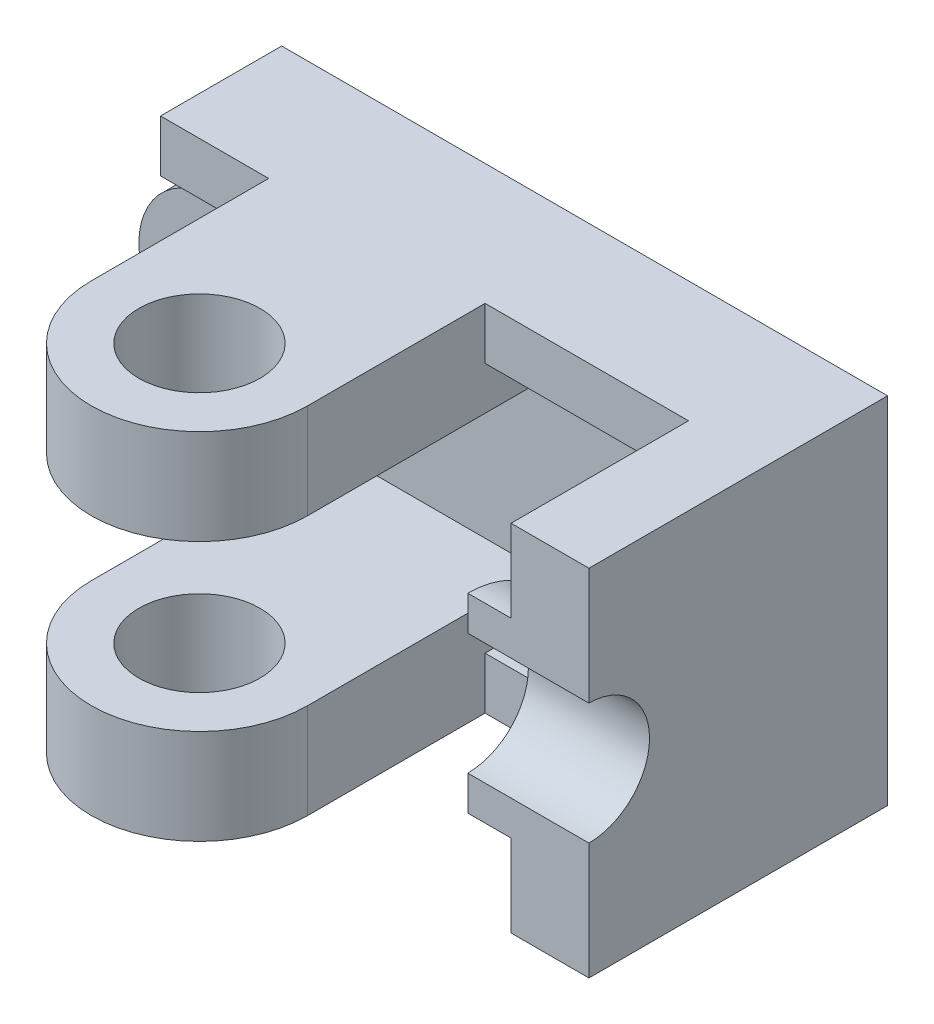
ISO-10303-21;
HEADER;
FILE_DESCRIPTION(('STEP AP214'),'2;1');
FILE_NAME('part.step','',(''),(''),'','','');
FILE_SCHEMA(('AUTOMOTIVE_DESIGN { 1 0 10303 214 1 1 1 1 }'));
ENDSEC;
DATA;
#1=APPLICATION_CONTEXT('core data for automotive mechanical design processes');
#2=APPLICATION_PROTOCOL_DEFINITION('international standard','automotive_design',2000,#1);
#3=PRODUCT_CONTEXT('',#1,'mechanical');
#4=PRODUCT('Part','Part','',(#3));
#5=PRODUCT_RELATED_PRODUCT_CATEGORY('part','',(#4));
#6=PRODUCT_DEFINITION_FORMATION('','',#4);
#7=PRODUCT_DEFINITION_CONTEXT('part definition',#1,'design');
#8=PRODUCT_DEFINITION('design','',#6,#7);
#9=PRODUCT_DEFINITION_SHAPE('','',#8);
#10=(LENGTH_UNIT() NAMED_UNIT(*) SI_UNIT(.MILLI.,.METRE.));
#11=(NAMED_UNIT(*) PLANE_ANGLE_UNIT() SI_UNIT($,.RADIAN.));
#12=(NAMED_UNIT(*) SI_UNIT($,.STERADIAN.) SOLID_ANGLE_UNIT());
#13=UNCERTAINTY_MEASURE_WITH_UNIT(LENGTH_MEASURE(1.E-05),#10,'distance_accuracy_value','');
#14=(GEOMETRIC_REPRESENTATION_CONTEXT(3) GLOBAL_UNCERTAINTY_ASSIGNED_CONTEXT((#13)) GLOBAL_UNIT_ASSIGNED_CONTEXT((#10,
#11,#12)) REPRESENTATION_CONTEXT('',''));
#15=CARTESIAN_POINT('',(0.,0.,0.));
#16=DIRECTION('',(0.,0.,1.));
#17=DIRECTION('',(1.,0.,0.));
#18=AXIS2_PLACEMENT_3D('',#15,#16,#17);
#19=CARTESIAN_POINT('',(0.,82.,15.));
#20=DIRECTION('',(1.,0.,0.));
#21=DIRECTION('',(0.,0.,-1.));
#22=AXIS2_PLACEMENT_3D('',#19,#20,#21);
#23=PLANE('',#22);
#24=DIRECTION('',(0.,-1.,0.));
#25=VECTOR('',#24,1.);
#26=CARTESIAN_POINT('',(0.,82.,0.));
#27=LINE('',#26,#25);
#28=CARTESIAN_POINT('',(0.,82.,0.));
#29=VERTEX_POINT('',#28);
#30=CARTESIAN_POINT('',(0.,59.,0.));
#31=VERTEX_POINT('',#30);
#32=EDGE_CURVE('E237',#29,#31,#27,.T.);
#33=ORIENTED_EDGE('',*,*,#32,.T.);
#34=DIRECTION('',(0.,0.,1.));
#35=VECTOR('',#34,1.);
#36=CARTESIAN_POINT('',(0.,59.,0.));
#37=LINE('',#36,#35);
#38=CARTESIAN_POINT('',(0.,59.,15.));
#39=VERTEX_POINT('',#38);
#40=EDGE_CURVE('E68',#31,#39,#37,.T.);
#41=ORIENTED_EDGE('',*,*,#40,.T.);
#42=DIRECTION('',(0.,-1.,0.));
#43=VECTOR('',#42,1.);
#44=CARTESIAN_POINT('',(0.,82.,15.));
#45=LINE('',#44,#43);
#46=CARTESIAN_POINT('',(0.,70.,15.));
#47=VERTEX_POINT('',#46);
#48=EDGE_CURVE('E439',#47,#39,#45,.T.);
#49=ORIENTED_EDGE('',*,*,#48,.F.);
#50=DIRECTION('',(0.,0.,1.));
#51=VECTOR('',#50,1.);
#52=CARTESIAN_POINT('',(0.,70.,28.));
#53=LINE('',#52,#51);
#54=CARTESIAN_POINT('',(0.,70.,28.));
#55=VERTEX_POINT('',#54);
#56=EDGE_CURVE('E257',#47,#55,#53,.T.);
#57=ORIENTED_EDGE('',*,*,#56,.T.);
#58=DIRECTION('',(0.,1.,0.));
#59=VECTOR('',#58,1.);
#60=CARTESIAN_POINT('',(0.,70.,28.));
#61=LINE('',#60,#59);
#62=CARTESIAN_POINT('',(0.,82.,28.));
#63=VERTEX_POINT('',#62);
#64=EDGE_CURVE('E269',#55,#63,#61,.T.);
#65=ORIENTED_EDGE('',*,*,#64,.T.);
#66=DIRECTION('',(0.,0.,-1.));
#67=VECTOR('',#66,1.);
#68=CARTESIAN_POINT('',(0.,82.,15.));
#69=LINE('',#68,#67);
#70=EDGE_CURVE('E441',#63,#29,#69,.T.);
#71=ORIENTED_EDGE('',*,*,#70,.T.);
#72=EDGE_LOOP('',(#33,#41,#49,#57,#65,#71));
#73=FACE_BOUND('',#72,.T.);
#74=ADVANCED_FACE('F44',(#73),#23,.F.);
#75=CARTESIAN_POINT('',(0.,0.,15.));
#76=DIRECTION('',(0.,0.,1.));
#77=DIRECTION('',(1.,0.,0.));
#78=AXIS2_PLACEMENT_3D('',#75,#76,#77);
#79=PLANE('',#78);
#80=CARTESIAN_POINT('',(0.,41.,15.));
#81=DIRECTION('',(0.,0.,1.));
#82=DIRECTION('',(1.,0.,0.));
#83=AXIS2_PLACEMENT_3D('',#80,#81,#82);
#84=CIRCLE('',#83,11.);
#85=CARTESIAN_POINT('',(11.,41.,15.));
#86=VERTEX_POINT('',#85);
#87=EDGE_CURVE('E254',#86,#86,#84,.T.);
#88=ORIENTED_EDGE('',*,*,#87,.F.);
#89=EDGE_LOOP('',(#88));
#90=FACE_BOUND('',#89,.T.);
#91=DIRECTION('',(-1.,0.,0.));
#92=VECTOR('',#91,1.);
#93=CARTESIAN_POINT('',(0.,70.,15.));
#94=LINE('',#93,#92);
#95=CARTESIAN_POINT('',(25.,70.,15.));
#96=VERTEX_POINT('',#95);
#97=EDGE_CURVE('E270',#96,#47,#94,.T.);
#98=ORIENTED_EDGE('',*,*,#97,.T.);
#99=ORIENTED_EDGE('',*,*,#48,.T.);
#100=CARTESIAN_POINT('',(0.,41.,15.));
#101=DIRECTION('',(0.,0.,1.));
#102=DIRECTION('',(1.,0.,0.));
#103=AXIS2_PLACEMENT_3D('',#100,#101,#102);
#104=CIRCLE('',#103,18.);
#105=CARTESIAN_POINT('',(0.,23.,15.));
#106=VERTEX_POINT('',#105);
#107=EDGE_CURVE('E247',#39,#106,#104,.T.);
#108=ORIENTED_EDGE('',*,*,#107,.T.);
#109=CARTESIAN_POINT('',(0.,12.,15.));
#110=VERTEX_POINT('',#109);
#111=EDGE_CURVE('E58',#106,#110,#45,.T.);
#112=ORIENTED_EDGE('',*,*,#111,.T.);
#113=DIRECTION('',(1.,0.,0.));
#114=VECTOR('',#113,1.);
#115=CARTESIAN_POINT('',(0.,12.,15.));
#116=LINE('',#115,#114);
#117=CARTESIAN_POINT('',(25.,12.,15.));
#118=VERTEX_POINT('',#117);
#119=EDGE_CURVE('E330',#110,#118,#116,.T.);
#120=ORIENTED_EDGE('',*,*,#119,.T.);
#121=DIRECTION('',(0.,-1.,0.));
#122=VECTOR('',#121,1.);
#123=CARTESIAN_POINT('',(25.,22.,15.));
#124=LINE('',#123,#122);
#125=CARTESIAN_POINT('',(25.,22.,15.));
#126=VERTEX_POINT('',#125);
#127=EDGE_CURVE('E395',#126,#118,#124,.T.);
#128=ORIENTED_EDGE('',*,*,#127,.F.);
#129=DIRECTION('',(1.,0.,0.));
#130=VECTOR('',#129,1.);
#131=CARTESIAN_POINT('',(75.,22.,15.));
#132=LINE('',#131,#130);
#133=CARTESIAN_POINT('',(75.,22.,15.));
#134=VERTEX_POINT('',#133);
#135=EDGE_CURVE('E373',#126,#134,#132,.T.);
#136=ORIENTED_EDGE('',*,*,#135,.T.);
#137=DIRECTION('',(0.,-1.,0.));
#138=VECTOR('',#137,1.);
#139=CARTESIAN_POINT('',(75.,22.,15.));
#140=LINE('',#139,#138);
#141=CARTESIAN_POINT('',(75.,12.,15.));
#142=VERTEX_POINT('',#141);
#143=EDGE_CURVE('E390',#134,#142,#140,.T.);
#144=ORIENTED_EDGE('',*,*,#143,.T.);
#145=DIRECTION('',(1.,0.,0.));
#146=VECTOR('',#145,1.);
#147=CARTESIAN_POINT('',(75.,12.,15.));
#148=LINE('',#147,#146);
#149=CARTESIAN_POINT('',(122.,12.,15.));
#150=VERTEX_POINT('',#149);
#151=EDGE_CURVE('E350',#142,#150,#148,.T.);
#152=ORIENTED_EDGE('',*,*,#151,.T.);
#153=DIRECTION('',(0.,1.,0.));
#154=VECTOR('',#153,1.);
#155=CARTESIAN_POINT('',(122.,0.,15.));
#156=LINE('',#155,#154);
#157=CARTESIAN_POINT('',(122.,70.,15.));
#158=VERTEX_POINT('',#157);
#159=EDGE_CURVE('E419',#150,#158,#156,.T.);
#160=ORIENTED_EDGE('',*,*,#159,.T.);
#161=DIRECTION('',(-1.,0.,0.));
#162=VECTOR('',#161,1.);
#163=CARTESIAN_POINT('',(75.,70.,15.));
#164=LINE('',#163,#162);
#165=CARTESIAN_POINT('',(75.,70.,15.));
#166=VERTEX_POINT('',#165);
#167=EDGE_CURVE('E308',#158,#166,#164,.T.);
#168=ORIENTED_EDGE('',*,*,#167,.T.);
#169=DIRECTION('',(0.,1.,0.));
#170=VECTOR('',#169,1.);
#171=CARTESIAN_POINT('',(75.,60.,15.));
#172=LINE('',#171,#170);
#173=CARTESIAN_POINT('',(75.,60.,15.));
#174=VERTEX_POINT('',#173);
#175=EDGE_CURVE('E301',#174,#166,#172,.T.);
#176=ORIENTED_EDGE('',*,*,#175,.F.);
#177=DIRECTION('',(-1.,0.,0.));
#178=VECTOR('',#177,1.);
#179=CARTESIAN_POINT('',(25.,60.,15.));
#180=LINE('',#179,#178);
#181=CARTESIAN_POINT('',(25.,60.,15.));
#182=VERTEX_POINT('',#181);
#183=EDGE_CURVE('E288',#174,#182,#180,.T.);
#184=ORIENTED_EDGE('',*,*,#183,.T.);
#185=DIRECTION('',(0.,1.,0.));
#186=VECTOR('',#185,1.);
#187=CARTESIAN_POINT('',(25.,60.,15.));
#188=LINE('',#187,#186);
#189=EDGE_CURVE('E300',#182,#96,#188,.T.);
#190=ORIENTED_EDGE('',*,*,#189,.T.);
#191=EDGE_LOOP('',(#98,#99,#108,#112,#120,#128,#136,#144,#152,#160,#168,#176,#184,#190));
#192=FACE_BOUND('',#191,.T.);
#193=ADVANCED_FACE('F535',(#90,#192),#79,.T.);
#194=CARTESIAN_POINT('',(122.,82.,69.));
#195=DIRECTION('',(0.,0.,1.));
#196=DIRECTION('',(1.,0.,0.));
#197=AXIS2_PLACEMENT_3D('',#194,#195,#196);
#198=PLANE('',#197);
#199=DIRECTION('',(-1.,0.,0.));
#200=VECTOR('',#199,1.);
#201=CARTESIAN_POINT('',(140.,55.,69.));
#202=LINE('',#201,#200);
#203=CARTESIAN_POINT('',(140.,55.,69.));
#204=VERTEX_POINT('',#203);
#205=CARTESIAN_POINT('',(112.,55.,69.));
#206=VERTEX_POINT('',#205);
#207=EDGE_CURVE('E402',#204,#206,#202,.T.);
#208=ORIENTED_EDGE('',*,*,#207,.F.);
#209=DIRECTION('',(0.,-1.,0.));
#210=VECTOR('',#209,1.);
#211=CARTESIAN_POINT('',(140.,82.,69.));
#212=LINE('',#211,#210);
#213=CARTESIAN_POINT('',(140.,82.,69.));
#214=VERTEX_POINT('',#213);
#215=EDGE_CURVE('E425',#214,#204,#212,.T.);
#216=ORIENTED_EDGE('',*,*,#215,.F.);
#217=DIRECTION('',(1.,0.,0.));
#218=VECTOR('',#217,1.);
#219=CARTESIAN_POINT('',(122.,82.,69.));
#220=LINE('',#219,#218);
#221=CARTESIAN_POINT('',(122.,82.,69.));
#222=VERTEX_POINT('',#221);
#223=EDGE_CURVE('E433',#222,#214,#220,.T.);
#224=ORIENTED_EDGE('',*,*,#223,.F.);
#225=DIRECTION('',(0.,-1.,0.));
#226=VECTOR('',#225,1.);
#227=CARTESIAN_POINT('',(122.,82.,69.));
#228=LINE('',#227,#226);
#229=CARTESIAN_POINT('',(122.,63.,69.));
#230=VERTEX_POINT('',#229);
#231=EDGE_CURVE('E430',#222,#230,#228,.T.);
#232=ORIENTED_EDGE('',*,*,#231,.T.);
#233=DIRECTION('',(1.,0.,0.));
#234=VECTOR('',#233,1.);
#235=CARTESIAN_POINT('',(112.,63.,69.));
#236=LINE('',#235,#234);
#237=CARTESIAN_POINT('',(112.,63.,69.));
#238=VERTEX_POINT('',#237);
#239=EDGE_CURVE('E413',#238,#230,#236,.T.);
#240=ORIENTED_EDGE('',*,*,#239,.F.);
#241=DIRECTION('',(0.,1.,0.));
#242=VECTOR('',#241,1.);
#243=CARTESIAN_POINT('',(112.,63.,69.));
#244=LINE('',#243,#242);
#245=EDGE_CURVE('E410',#206,#238,#244,.T.);
#246=ORIENTED_EDGE('',*,*,#245,.F.);
#247=EDGE_LOOP('',(#208,#216,#224,#232,#240,#246));
#248=FACE_BOUND('',#247,.T.);
#249=ADVANCED_FACE('F492',(#248),#198,.T.);
#250=CARTESIAN_POINT('',(122.,0.,0.));
#251=DIRECTION('',(1.,0.,0.));
#252=DIRECTION('',(0.,0.,-1.));
#253=AXIS2_PLACEMENT_3D('',#250,#251,#252);
#254=PLANE('',#253);
#255=DIRECTION('',(0.,0.,1.));
#256=VECTOR('',#255,1.);
#257=CARTESIAN_POINT('',(122.,82.,15.));
#258=LINE('',#257,#256);
#259=CARTESIAN_POINT('',(122.,82.,28.));
#260=VERTEX_POINT('',#259);
#261=EDGE_CURVE('E421',#260,#222,#258,.T.);
#262=ORIENTED_EDGE('',*,*,#261,.F.);
#263=DIRECTION('',(0.,1.,0.));
#264=VECTOR('',#263,1.);
#265=CARTESIAN_POINT('',(122.,70.,28.));
#266=LINE('',#265,#264);
#267=CARTESIAN_POINT('',(122.,70.,28.));
#268=VERTEX_POINT('',#267);
#269=EDGE_CURVE('E323',#268,#260,#266,.T.);
#270=ORIENTED_EDGE('',*,*,#269,.F.);
#271=DIRECTION('',(0.,0.,-1.));
#272=VECTOR('',#271,1.);
#273=CARTESIAN_POINT('',(122.,70.,15.));
#274=LINE('',#273,#272);
#275=EDGE_CURVE('E317',#268,#158,#274,.T.);
#276=ORIENTED_EDGE('',*,*,#275,.T.);
#277=ORIENTED_EDGE('',*,*,#159,.F.);
#278=DIRECTION('',(0.,0.,1.));
#279=VECTOR('',#278,1.);
#280=CARTESIAN_POINT('',(122.,12.,15.));
#281=LINE('',#280,#279);
#282=CARTESIAN_POINT('',(122.,12.,28.));
#283=VERTEX_POINT('',#282);
#284=EDGE_CURVE('E349',#150,#283,#281,.T.);
#285=ORIENTED_EDGE('',*,*,#284,.T.);
#286=DIRECTION('',(0.,-1.,0.));
#287=VECTOR('',#286,1.);
#288=CARTESIAN_POINT('',(122.,12.,28.));
#289=LINE('',#288,#287);
#290=CARTESIAN_POINT('',(122.,0.,28.));
#291=VERTEX_POINT('',#290);
#292=EDGE_CURVE('E356',#283,#291,#289,.T.);
#293=ORIENTED_EDGE('',*,*,#292,.T.);
#294=DIRECTION('',(0.,0.,-1.));
#295=VECTOR('',#294,1.);
#296=CARTESIAN_POINT('',(122.,0.,69.));
#297=LINE('',#296,#295);
#298=CARTESIAN_POINT('',(122.,0.,69.));
#299=VERTEX_POINT('',#298);
#300=EDGE_CURVE('E427',#299,#291,#297,.T.);
#301=ORIENTED_EDGE('',*,*,#300,.F.);
#302=CARTESIAN_POINT('',(122.,19.,69.));
#303=VERTEX_POINT('',#302);
#304=EDGE_CURVE('E428',#303,#299,#228,.T.);
#305=ORIENTED_EDGE('',*,*,#304,.F.);
#306=CARTESIAN_POINT('',(122.,41.,69.));
#307=DIRECTION('',(-1.,0.,0.));
#308=DIRECTION('',(0.,0.,1.));
#309=AXIS2_PLACEMENT_3D('',#306,#307,#308);
#310=CIRCLE('',#309,22.);
#311=EDGE_CURVE('E401',#230,#303,#310,.T.);
#312=ORIENTED_EDGE('',*,*,#311,.F.);
#313=ORIENTED_EDGE('',*,*,#231,.F.);
#314=EDGE_LOOP('',(#262,#270,#276,#277,#285,#293,#301,#305,#312,#313));
#315=FACE_BOUND('',#314,.T.);
#316=ADVANCED_FACE('F490',(#315),#254,.F.);
#317=ORIENTED_EDGE('',*,*,#111,.F.);
#318=DIRECTION('',(0.,0.,1.));
#319=VECTOR('',#318,1.);
#320=CARTESIAN_POINT('',(0.,23.,0.));
#321=LINE('',#320,#319);
#322=CARTESIAN_POINT('',(0.,23.,0.));
#323=VERTEX_POINT('',#322);
#324=EDGE_CURVE('E245',#323,#106,#321,.T.);
#325=ORIENTED_EDGE('',*,*,#324,.F.);
#326=CARTESIAN_POINT('',(0.,0.,0.));
#327=VERTEX_POINT('',#326);
#328=EDGE_CURVE('E235',#323,#327,#27,.T.);
#329=ORIENTED_EDGE('',*,*,#328,.T.);
#330=DIRECTION('',(0.,0.,-1.));
#331=VECTOR('',#330,1.);
#332=CARTESIAN_POINT('',(0.,0.,15.));
#333=LINE('',#332,#331);
#334=CARTESIAN_POINT('',(0.,0.,28.));
#335=VERTEX_POINT('',#334);
#336=EDGE_CURVE('E11',#335,#327,#333,.T.);
#337=ORIENTED_EDGE('',*,*,#336,.F.);
#338=DIRECTION('',(0.,-1.,0.));
#339=VECTOR('',#338,1.);
#340=CARTESIAN_POINT('',(0.,12.,28.));
#341=LINE('',#340,#339);
#342=CARTESIAN_POINT('',(0.,12.,28.));
#343=VERTEX_POINT('',#342);
#344=EDGE_CURVE('E343',#343,#335,#341,.T.);
#345=ORIENTED_EDGE('',*,*,#344,.F.);
#346=DIRECTION('',(0.,0.,-1.));
#347=VECTOR('',#346,1.);
#348=CARTESIAN_POINT('',(0.,12.,28.));
#349=LINE('',#348,#347);
#350=EDGE_CURVE('E337',#343,#110,#349,.T.);
#351=ORIENTED_EDGE('',*,*,#350,.T.);
#352=EDGE_LOOP('',(#317,#325,#329,#337,#345,#351));
#353=FACE_BOUND('',#352,.T.);
#354=ADVANCED_FACE('F50',(#353),#23,.F.);
#355=CARTESIAN_POINT('',(0.,0.,15.));
#356=DIRECTION('',(0.,1.,0.));
#357=DIRECTION('',(0.,0.,1.));
#358=AXIS2_PLACEMENT_3D('',#355,#356,#357);
#359=PLANE('',#358);
#360=CARTESIAN_POINT('',(50.,0.,69.));
#361=DIRECTION('',(0.,-1.,0.));
#362=DIRECTION('',(0.,0.,-1.));
#363=AXIS2_PLACEMENT_3D('',#360,#361,#362);
#364=CIRCLE('',#363,14.);
#365=CARTESIAN_POINT('',(50.,0.,55.));
#366=VERTEX_POINT('',#365);
#367=EDGE_CURVE('E958',#366,#366,#364,.T.);
#368=ORIENTED_EDGE('',*,*,#367,.F.);
#369=EDGE_LOOP('',(#368));
#370=FACE_BOUND('',#369,.T.);
#371=ORIENTED_EDGE('',*,*,#300,.T.);
#372=DIRECTION('',(-1.,0.,0.));
#373=VECTOR('',#372,1.);
#374=CARTESIAN_POINT('',(122.,0.,28.));
#375=LINE('',#374,#373);
#376=CARTESIAN_POINT('',(75.,0.,28.));
#377=VERTEX_POINT('',#376);
#378=EDGE_CURVE('E345',#291,#377,#375,.T.);
#379=ORIENTED_EDGE('',*,*,#378,.T.);
#380=DIRECTION('',(0.,0.,1.));
#381=VECTOR('',#380,1.);
#382=CARTESIAN_POINT('',(75.,0.,69.));
#383=LINE('',#382,#381);
#384=CARTESIAN_POINT('',(75.,0.,69.));
#385=VERTEX_POINT('',#384);
#386=EDGE_CURVE('E369',#377,#385,#383,.T.);
#387=ORIENTED_EDGE('',*,*,#386,.T.);
#388=CARTESIAN_POINT('',(50.,0.,69.));
#389=DIRECTION('',(0.,-1.,0.));
#390=DIRECTION('',(0.,0.,-1.));
#391=AXIS2_PLACEMENT_3D('',#388,#389,#390);
#392=CIRCLE('',#391,25.);
#393=CARTESIAN_POINT('',(25.,0.,69.));
#394=VERTEX_POINT('',#393);
#395=EDGE_CURVE('E361',#385,#394,#392,.T.);
#396=ORIENTED_EDGE('',*,*,#395,.T.);
#397=DIRECTION('',(0.,0.,-1.));
#398=VECTOR('',#397,1.);
#399=CARTESIAN_POINT('',(25.,0.,69.));
#400=LINE('',#399,#398);
#401=CARTESIAN_POINT('',(25.,0.,28.));
#402=VERTEX_POINT('',#401);
#403=EDGE_CURVE('E382',#394,#402,#400,.T.);
#404=ORIENTED_EDGE('',*,*,#403,.T.);
#405=DIRECTION('',(-1.,0.,0.));
#406=VECTOR('',#405,1.);
#407=CARTESIAN_POINT('',(25.,0.,28.));
#408=LINE('',#407,#406);
#409=EDGE_CURVE('E325',#402,#335,#408,.T.);
#410=ORIENTED_EDGE('',*,*,#409,.T.);
#411=ORIENTED_EDGE('',*,*,#336,.T.);
#412=DIRECTION('',(1.,0.,0.));
#413=VECTOR('',#412,1.);
#414=CARTESIAN_POINT('',(0.,0.,0.));
#415=LINE('',#414,#413);
#416=CARTESIAN_POINT('',(140.,0.,0.));
#417=VERTEX_POINT('',#416);
#418=EDGE_CURVE('E238',#327,#417,#415,.T.);
#419=ORIENTED_EDGE('',*,*,#418,.T.);
#420=DIRECTION('',(0.,0.,-1.));
#421=VECTOR('',#420,1.);
#422=CARTESIAN_POINT('',(140.,0.,15.));
#423=LINE('',#422,#421);
#424=CARTESIAN_POINT('',(140.,0.,69.));
#425=VERTEX_POINT('',#424);
#426=EDGE_CURVE('E52',#425,#417,#423,.T.);
#427=ORIENTED_EDGE('',*,*,#426,.F.);
#428=DIRECTION('',(1.,0.,0.));
#429=VECTOR('',#428,1.);
#430=CARTESIAN_POINT('',(122.,0.,69.));
#431=LINE('',#430,#429);
#432=EDGE_CURVE('E239',#299,#425,#431,.T.);
#433=ORIENTED_EDGE('',*,*,#432,.F.);
#434=EDGE_LOOP('',(#371,#379,#387,#396,#404,#410,#411,#419,#427,#433));
#435=FACE_BOUND('',#434,.T.);
#436=ADVANCED_FACE('F503',(#370,#435),#359,.F.);
#437=CARTESIAN_POINT('',(140.,0.,15.));
#438=DIRECTION('',(-1.,0.,0.));
#439=DIRECTION('',(0.,0.,1.));
#440=AXIS2_PLACEMENT_3D('',#437,#438,#439);
#441=PLANE('',#440);
#442=ORIENTED_EDGE('',*,*,#215,.T.);
#443=CARTESIAN_POINT('',(140.,41.,69.));
#444=DIRECTION('',(-1.,0.,0.));
#445=DIRECTION('',(0.,0.,1.));
#446=AXIS2_PLACEMENT_3D('',#443,#444,#445);
#447=CIRCLE('',#446,14.);
#448=CARTESIAN_POINT('',(140.,27.,69.));
#449=VERTEX_POINT('',#448);
#450=EDGE_CURVE('E396',#204,#449,#447,.T.);
#451=ORIENTED_EDGE('',*,*,#450,.T.);
#452=EDGE_CURVE('E417',#449,#425,#212,.T.);
#453=ORIENTED_EDGE('',*,*,#452,.T.);
#454=ORIENTED_EDGE('',*,*,#426,.T.);
#455=DIRECTION('',(0.,1.,0.));
#456=VECTOR('',#455,1.);
#457=CARTESIAN_POINT('',(140.,0.,0.));
#458=LINE('',#457,#456);
#459=CARTESIAN_POINT('',(140.,82.,0.));
#460=VERTEX_POINT('',#459);
#461=EDGE_CURVE('E443',#417,#460,#458,.T.);
#462=ORIENTED_EDGE('',*,*,#461,.T.);
#463=DIRECTION('',(0.,0.,-1.));
#464=VECTOR('',#463,1.);
#465=CARTESIAN_POINT('',(140.,82.,15.));
#466=LINE('',#465,#464);
#467=EDGE_CURVE('E448',#214,#460,#466,.T.);
#468=ORIENTED_EDGE('',*,*,#467,.F.);
#469=EDGE_LOOP('',(#442,#451,#453,#454,#462,#468));
#470=FACE_BOUND('',#469,.T.);
#471=ADVANCED_FACE('F451',(#470),#441,.F.);
#472=CARTESIAN_POINT('',(140.,82.,15.));
#473=DIRECTION('',(0.,-1.,0.));
#474=DIRECTION('',(0.,0.,-1.));
#475=AXIS2_PLACEMENT_3D('',#472,#473,#474);
#476=PLANE('',#475);
#477=CARTESIAN_POINT('',(50.,82.,69.));
#478=DIRECTION('',(0.,1.,0.));
#479=DIRECTION('',(0.,0.,1.));
#480=AXIS2_PLACEMENT_3D('',#477,#478,#479);
#481=CIRCLE('',#480,14.);
#482=CARTESIAN_POINT('',(50.,82.,83.));
#483=VERTEX_POINT('',#482);
#484=EDGE_CURVE('E951',#483,#483,#481,.T.);
#485=ORIENTED_EDGE('',*,*,#484,.F.);
#486=EDGE_LOOP('',(#485));
#487=FACE_BOUND('',#486,.T.);
#488=ORIENTED_EDGE('',*,*,#70,.F.);
#489=DIRECTION('',(1.,0.,0.));
#490=VECTOR('',#489,1.);
#491=CARTESIAN_POINT('',(25.,82.,28.));
#492=LINE('',#491,#490);
#493=CARTESIAN_POINT('',(25.,82.,28.));
#494=VERTEX_POINT('',#493);
#495=EDGE_CURVE('E258',#63,#494,#492,.T.);
#496=ORIENTED_EDGE('',*,*,#495,.T.);
#497=DIRECTION('',(0.,0.,1.));
#498=VECTOR('',#497,1.);
#499=CARTESIAN_POINT('',(25.,82.,69.));
#500=LINE('',#499,#498);
#501=CARTESIAN_POINT('',(25.,82.,69.));
#502=VERTEX_POINT('',#501);
#503=EDGE_CURVE('E273',#494,#502,#500,.T.);
#504=ORIENTED_EDGE('',*,*,#503,.T.);
#505=CARTESIAN_POINT('',(50.,82.,69.));
#506=DIRECTION('',(0.,1.,0.));
#507=DIRECTION('',(0.,0.,1.));
#508=AXIS2_PLACEMENT_3D('',#505,#506,#507);
#509=CIRCLE('',#508,25.);
#510=CARTESIAN_POINT('',(75.,82.,69.));
#511=VERTEX_POINT('',#510);
#512=EDGE_CURVE('E292',#502,#511,#509,.T.);
#513=ORIENTED_EDGE('',*,*,#512,.T.);
#514=DIRECTION('',(0.,0.,-1.));
#515=VECTOR('',#514,1.);
#516=CARTESIAN_POINT('',(75.,82.,15.));
#517=LINE('',#516,#515);
#518=CARTESIAN_POINT('',(75.,82.,28.));
#519=VERTEX_POINT('',#518);
#520=EDGE_CURVE('E285',#511,#519,#517,.T.);
#521=ORIENTED_EDGE('',*,*,#520,.T.);
#522=DIRECTION('',(1.,0.,0.));
#523=VECTOR('',#522,1.);
#524=CARTESIAN_POINT('',(122.,82.,28.));
#525=LINE('',#524,#523);
#526=EDGE_CURVE('E297',#519,#260,#525,.T.);
#527=ORIENTED_EDGE('',*,*,#526,.T.);
#528=ORIENTED_EDGE('',*,*,#261,.T.);
#529=ORIENTED_EDGE('',*,*,#223,.T.);
#530=ORIENTED_EDGE('',*,*,#467,.T.);
#531=DIRECTION('',(-1.,0.,0.));
#532=VECTOR('',#531,1.);
#533=CARTESIAN_POINT('',(140.,82.,0.));
#534=LINE('',#533,#532);
#535=EDGE_CURVE('E447',#460,#29,#534,.T.);
#536=ORIENTED_EDGE('',*,*,#535,.T.);
#537=EDGE_LOOP('',(#488,#496,#504,#513,#521,#527,#528,#529,#530,#536));
#538=FACE_BOUND('',#537,.T.);
#539=ADVANCED_FACE('F461',(#487,#538),#476,.F.);
#540=CARTESIAN_POINT('',(0.,0.,0.));
#541=DIRECTION('',(0.,0.,1.));
#542=DIRECTION('',(1.,0.,0.));
#543=AXIS2_PLACEMENT_3D('',#540,#541,#542);
#544=PLANE('',#543);
#545=CARTESIAN_POINT('',(0.,41.,0.));
#546=DIRECTION('',(0.,0.,1.));
#547=DIRECTION('',(1.,0.,0.));
#548=AXIS2_PLACEMENT_3D('',#545,#546,#547);
#549=CIRCLE('',#548,11.);
#550=CARTESIAN_POINT('',(11.,41.,0.));
#551=VERTEX_POINT('',#550);
#552=EDGE_CURVE('E249',#551,#551,#549,.T.);
#553=ORIENTED_EDGE('',*,*,#552,.T.);
#554=EDGE_LOOP('',(#553));
#555=FACE_BOUND('',#554,.T.);
#556=ORIENTED_EDGE('',*,*,#32,.F.);
#557=ORIENTED_EDGE('',*,*,#535,.F.);
#558=ORIENTED_EDGE('',*,*,#461,.F.);
#559=ORIENTED_EDGE('',*,*,#418,.F.);
#560=ORIENTED_EDGE('',*,*,#328,.F.);
#561=CARTESIAN_POINT('',(0.,41.,0.));
#562=DIRECTION('',(0.,0.,1.));
#563=DIRECTION('',(1.,0.,0.));
#564=AXIS2_PLACEMENT_3D('',#561,#562,#563);
#565=CIRCLE('',#564,18.);
#566=EDGE_CURVE('E236',#31,#323,#565,.T.);
#567=ORIENTED_EDGE('',*,*,#566,.F.);
#568=EDGE_LOOP('',(#556,#557,#558,#559,#560,#567));
#569=FACE_BOUND('',#568,.T.);
#570=ADVANCED_FACE('F234',(#555,#569),#544,.F.);
#571=DIRECTION('',(-1.,0.,0.));
#572=VECTOR('',#571,1.);
#573=CARTESIAN_POINT('',(140.,27.,69.));
#574=LINE('',#573,#572);
#575=CARTESIAN_POINT('',(112.,27.,69.));
#576=VERTEX_POINT('',#575);
#577=EDGE_CURVE('E397',#449,#576,#574,.T.);
#578=ORIENTED_EDGE('',*,*,#577,.T.);
#579=CARTESIAN_POINT('',(112.,19.,69.));
#580=VERTEX_POINT('',#579);
#581=EDGE_CURVE('E406',#580,#576,#244,.T.);
#582=ORIENTED_EDGE('',*,*,#581,.F.);
#583=DIRECTION('',(1.,0.,0.));
#584=VECTOR('',#583,1.);
#585=CARTESIAN_POINT('',(112.,19.,69.));
#586=LINE('',#585,#584);
#587=EDGE_CURVE('E416',#580,#303,#586,.T.);
#588=ORIENTED_EDGE('',*,*,#587,.T.);
#589=ORIENTED_EDGE('',*,*,#304,.T.);
#590=ORIENTED_EDGE('',*,*,#432,.T.);
#591=ORIENTED_EDGE('',*,*,#452,.F.);
#592=EDGE_LOOP('',(#578,#582,#588,#589,#590,#591));
#593=FACE_BOUND('',#592,.T.);
#594=ADVANCED_FACE('F501',(#593),#198,.T.);
#595=CARTESIAN_POINT('',(112.,41.,69.));
#596=DIRECTION('',(1.,0.,0.));
#597=DIRECTION('',(0.,0.,-1.));
#598=AXIS2_PLACEMENT_3D('',#595,#596,#597);
#599=CYLINDRICAL_SURFACE('',#598,22.);
#600=ORIENTED_EDGE('',*,*,#311,.T.);
#601=ORIENTED_EDGE('',*,*,#587,.F.);
#602=CARTESIAN_POINT('',(112.,41.,69.));
#603=DIRECTION('',(-1.,0.,0.));
#604=DIRECTION('',(0.,0.,1.));
#605=AXIS2_PLACEMENT_3D('',#602,#603,#604);
#606=CIRCLE('',#605,22.);
#607=EDGE_CURVE('E408',#238,#580,#606,.T.);
#608=ORIENTED_EDGE('',*,*,#607,.F.);
#609=ORIENTED_EDGE('',*,*,#239,.T.);
#610=EDGE_LOOP('',(#600,#601,#608,#609));
#611=FACE_BOUND('',#610,.T.);
#612=ADVANCED_FACE('F572',(#611),#599,.T.);
#613=CARTESIAN_POINT('',(112.,41.,69.));
#614=DIRECTION('',(-1.,0.,0.));
#615=DIRECTION('',(0.,0.,1.));
#616=AXIS2_PLACEMENT_3D('',#613,#614,#615);
#617=PLANE('',#616);
#618=CARTESIAN_POINT('',(112.,41.,69.));
#619=DIRECTION('',(-1.,0.,0.));
#620=DIRECTION('',(0.,0.,1.));
#621=AXIS2_PLACEMENT_3D('',#618,#619,#620);
#622=CIRCLE('',#621,14.);
#623=EDGE_CURVE('E387',#206,#576,#622,.T.);
#624=ORIENTED_EDGE('',*,*,#623,.F.);
#625=ORIENTED_EDGE('',*,*,#245,.T.);
#626=ORIENTED_EDGE('',*,*,#607,.T.);
#627=ORIENTED_EDGE('',*,*,#581,.T.);
#628=EDGE_LOOP('',(#624,#625,#626,#627));
#629=FACE_BOUND('',#628,.T.);
#630=ADVANCED_FACE('F607',(#629),#617,.T.);
#631=CARTESIAN_POINT('',(140.,41.,69.));
#632=DIRECTION('',(-1.,0.,0.));
#633=DIRECTION('',(0.,0.,1.));
#634=AXIS2_PLACEMENT_3D('',#631,#632,#633);
#635=CYLINDRICAL_SURFACE('',#634,14.);
#636=ORIENTED_EDGE('',*,*,#623,.T.);
#637=ORIENTED_EDGE('',*,*,#577,.F.);
#638=ORIENTED_EDGE('',*,*,#450,.F.);
#639=ORIENTED_EDGE('',*,*,#207,.T.);
#640=EDGE_LOOP('',(#636,#637,#638,#639));
#641=FACE_BOUND('',#640,.T.);
#642=ADVANCED_FACE('F614',(#641),#635,.F.);
#643=CARTESIAN_POINT('',(50.,22.,69.));
#644=DIRECTION('',(0.,-1.,0.));
#645=DIRECTION('',(0.,0.,-1.));
#646=AXIS2_PLACEMENT_3D('',#643,#644,#645);
#647=CYLINDRICAL_SURFACE('',#646,25.);
#648=ORIENTED_EDGE('',*,*,#395,.F.);
#649=DIRECTION('',(0.,-1.,0.));
#650=VECTOR('',#649,1.);
#651=CARTESIAN_POINT('',(75.,22.,69.));
#652=LINE('',#651,#650);
#653=CARTESIAN_POINT('',(75.,22.,69.));
#654=VERTEX_POINT('',#653);
#655=EDGE_CURVE('E383',#654,#385,#652,.T.);
#656=ORIENTED_EDGE('',*,*,#655,.F.);
#657=CARTESIAN_POINT('',(50.,22.,69.));
#658=DIRECTION('',(0.,-1.,0.));
#659=DIRECTION('',(0.,0.,-1.));
#660=AXIS2_PLACEMENT_3D('',#657,#658,#659);
#661=CIRCLE('',#660,25.);
#662=CARTESIAN_POINT('',(25.,22.,69.));
#663=VERTEX_POINT('',#662);
#664=EDGE_CURVE('E366',#654,#663,#661,.T.);
#665=ORIENTED_EDGE('',*,*,#664,.T.);
#666=DIRECTION('',(0.,-1.,0.));
#667=VECTOR('',#666,1.);
#668=CARTESIAN_POINT('',(25.,22.,69.));
#669=LINE('',#668,#667);
#670=EDGE_CURVE('E377',#663,#394,#669,.T.);
#671=ORIENTED_EDGE('',*,*,#670,.T.);
#672=EDGE_LOOP('',(#648,#656,#665,#671));
#673=FACE_BOUND('',#672,.T.);
#674=ADVANCED_FACE('F520',(#673),#647,.T.);
#675=CARTESIAN_POINT('',(75.,22.,69.));
#676=DIRECTION('',(1.,0.,0.));
#677=DIRECTION('',(0.,0.,-1.));
#678=AXIS2_PLACEMENT_3D('',#675,#676,#677);
#679=PLANE('',#678);
#680=DIRECTION('',(0.,-1.,0.));
#681=VECTOR('',#680,1.);
#682=CARTESIAN_POINT('',(75.,12.,28.));
#683=LINE('',#682,#681);
#684=CARTESIAN_POINT('',(75.,12.,28.));
#685=VERTEX_POINT('',#684);
#686=EDGE_CURVE('E359',#685,#377,#683,.T.);
#687=ORIENTED_EDGE('',*,*,#686,.F.);
#688=DIRECTION('',(0.,0.,-1.));
#689=VECTOR('',#688,1.);
#690=CARTESIAN_POINT('',(75.,12.,28.));
#691=LINE('',#690,#689);
#692=EDGE_CURVE('E354',#685,#142,#691,.T.);
#693=ORIENTED_EDGE('',*,*,#692,.T.);
#694=ORIENTED_EDGE('',*,*,#143,.F.);
#695=DIRECTION('',(0.,0.,1.));
#696=VECTOR('',#695,1.);
#697=CARTESIAN_POINT('',(75.,22.,69.));
#698=LINE('',#697,#696);
#699=EDGE_CURVE('E374',#134,#654,#698,.T.);
#700=ORIENTED_EDGE('',*,*,#699,.T.);
#701=ORIENTED_EDGE('',*,*,#655,.T.);
#702=ORIENTED_EDGE('',*,*,#386,.F.);
#703=EDGE_LOOP('',(#687,#693,#694,#700,#701,#702));
#704=FACE_BOUND('',#703,.T.);
#705=ADVANCED_FACE('F513',(#704),#679,.T.);
#706=CARTESIAN_POINT('',(25.,22.,69.));
#707=DIRECTION('',(-1.,0.,0.));
#708=DIRECTION('',(0.,0.,1.));
#709=AXIS2_PLACEMENT_3D('',#706,#707,#708);
#710=PLANE('',#709);
#711=DIRECTION('',(0.,-1.,0.));
#712=VECTOR('',#711,1.);
#713=CARTESIAN_POINT('',(25.,12.,28.));
#714=LINE('',#713,#712);
#715=CARTESIAN_POINT('',(25.,12.,28.));
#716=VERTEX_POINT('',#715);
#717=EDGE_CURVE('E336',#716,#402,#714,.T.);
#718=ORIENTED_EDGE('',*,*,#717,.T.);
#719=ORIENTED_EDGE('',*,*,#403,.F.);
#720=ORIENTED_EDGE('',*,*,#670,.F.);
#721=DIRECTION('',(0.,0.,-1.));
#722=VECTOR('',#721,1.);
#723=CARTESIAN_POINT('',(25.,22.,69.));
#724=LINE('',#723,#722);
#725=EDGE_CURVE('E367',#663,#126,#724,.T.);
#726=ORIENTED_EDGE('',*,*,#725,.T.);
#727=ORIENTED_EDGE('',*,*,#127,.T.);
#728=DIRECTION('',(0.,0.,1.));
#729=VECTOR('',#728,1.);
#730=CARTESIAN_POINT('',(25.,12.,15.));
#731=LINE('',#730,#729);
#732=EDGE_CURVE('E329',#118,#716,#731,.T.);
#733=ORIENTED_EDGE('',*,*,#732,.T.);
#734=EDGE_LOOP('',(#718,#719,#720,#726,#727,#733));
#735=FACE_BOUND('',#734,.T.);
#736=ADVANCED_FACE('F523',(#735),#710,.T.);
#737=CARTESIAN_POINT('',(50.,22.,69.));
#738=DIRECTION('',(0.,-1.,0.));
#739=DIRECTION('',(0.,0.,-1.));
#740=AXIS2_PLACEMENT_3D('',#737,#738,#739);
#741=PLANE('',#740);
#742=CARTESIAN_POINT('',(50.,22.,69.));
#743=DIRECTION('',(0.,-1.,0.));
#744=DIRECTION('',(0.,0.,-1.));
#745=AXIS2_PLACEMENT_3D('',#742,#743,#744);
#746=CIRCLE('',#745,14.);
#747=CARTESIAN_POINT('',(50.,22.,55.));
#748=VERTEX_POINT('',#747);
#749=EDGE_CURVE('E954',#748,#748,#746,.T.);
#750=ORIENTED_EDGE('',*,*,#749,.T.);
#751=EDGE_LOOP('',(#750));
#752=FACE_BOUND('',#751,.T.);
#753=ORIENTED_EDGE('',*,*,#664,.F.);
#754=ORIENTED_EDGE('',*,*,#699,.F.);
#755=ORIENTED_EDGE('',*,*,#135,.F.);
#756=ORIENTED_EDGE('',*,*,#725,.F.);
#757=EDGE_LOOP('',(#753,#754,#755,#756));
#758=FACE_BOUND('',#757,.T.);
#759=ADVANCED_FACE('F533',(#752,#758),#741,.F.);
#760=CARTESIAN_POINT('',(122.,12.,28.));
#761=DIRECTION('',(0.,0.,1.));
#762=DIRECTION('',(1.,0.,0.));
#763=AXIS2_PLACEMENT_3D('',#760,#761,#762);
#764=PLANE('',#763);
#765=ORIENTED_EDGE('',*,*,#378,.F.);
#766=ORIENTED_EDGE('',*,*,#292,.F.);
#767=DIRECTION('',(-1.,0.,0.));
#768=VECTOR('',#767,1.);
#769=CARTESIAN_POINT('',(122.,12.,28.));
#770=LINE('',#769,#768);
#771=EDGE_CURVE('E353',#283,#685,#770,.T.);
#772=ORIENTED_EDGE('',*,*,#771,.T.);
#773=ORIENTED_EDGE('',*,*,#686,.T.);
#774=EDGE_LOOP('',(#765,#766,#772,#773));
#775=FACE_BOUND('',#774,.T.);
#776=ADVANCED_FACE('F510',(#775),#764,.T.);
#777=CARTESIAN_POINT('',(0.,12.,0.));
#778=DIRECTION('',(0.,-1.,0.));
#779=DIRECTION('',(0.,0.,-1.));
#780=AXIS2_PLACEMENT_3D('',#777,#778,#779);
#781=PLANE('',#780);
#782=ORIENTED_EDGE('',*,*,#151,.F.);
#783=ORIENTED_EDGE('',*,*,#692,.F.);
#784=ORIENTED_EDGE('',*,*,#771,.F.);
#785=ORIENTED_EDGE('',*,*,#284,.F.);
#786=EDGE_LOOP('',(#782,#783,#784,#785));
#787=FACE_BOUND('',#786,.T.);
#788=ADVANCED_FACE('F509',(#787),#781,.F.);
#789=CARTESIAN_POINT('',(25.,12.,28.));
#790=DIRECTION('',(0.,0.,1.));
#791=DIRECTION('',(1.,0.,0.));
#792=AXIS2_PLACEMENT_3D('',#789,#790,#791);
#793=PLANE('',#792);
#794=ORIENTED_EDGE('',*,*,#409,.F.);
#795=ORIENTED_EDGE('',*,*,#717,.F.);
#796=DIRECTION('',(-1.,0.,0.));
#797=VECTOR('',#796,1.);
#798=CARTESIAN_POINT('',(25.,12.,28.));
#799=LINE('',#798,#797);
#800=EDGE_CURVE('E333',#716,#343,#799,.T.);
#801=ORIENTED_EDGE('',*,*,#800,.T.);
#802=ORIENTED_EDGE('',*,*,#344,.T.);
#803=EDGE_LOOP('',(#794,#795,#801,#802));
#804=FACE_BOUND('',#803,.T.);
#805=ADVANCED_FACE('F526',(#804),#793,.T.);
#806=CARTESIAN_POINT('',(0.,12.,0.));
#807=DIRECTION('',(0.,-1.,0.));
#808=DIRECTION('',(0.,0.,-1.));
#809=AXIS2_PLACEMENT_3D('',#806,#807,#808);
#810=PLANE('',#809);
#811=ORIENTED_EDGE('',*,*,#119,.F.);
#812=ORIENTED_EDGE('',*,*,#350,.F.);
#813=ORIENTED_EDGE('',*,*,#800,.F.);
#814=ORIENTED_EDGE('',*,*,#732,.F.);
#815=EDGE_LOOP('',(#811,#812,#813,#814));
#816=FACE_BOUND('',#815,.T.);
#817=ADVANCED_FACE('F529',(#816),#810,.F.);
#818=CARTESIAN_POINT('',(122.,70.,28.));
#819=DIRECTION('',(0.,0.,1.));
#820=DIRECTION('',(1.,0.,0.));
#821=AXIS2_PLACEMENT_3D('',#818,#819,#820);
#822=PLANE('',#821);
#823=ORIENTED_EDGE('',*,*,#526,.F.);
#824=DIRECTION('',(0.,1.,0.));
#825=VECTOR('',#824,1.);
#826=CARTESIAN_POINT('',(75.,70.,28.));
#827=LINE('',#826,#825);
#828=CARTESIAN_POINT('',(75.,70.,28.));
#829=VERTEX_POINT('',#828);
#830=EDGE_CURVE('E316',#829,#519,#827,.T.);
#831=ORIENTED_EDGE('',*,*,#830,.F.);
#832=DIRECTION('',(1.,0.,0.));
#833=VECTOR('',#832,1.);
#834=CARTESIAN_POINT('',(122.,70.,28.));
#835=LINE('',#834,#833);
#836=EDGE_CURVE('E313',#829,#268,#835,.T.);
#837=ORIENTED_EDGE('',*,*,#836,.T.);
#838=ORIENTED_EDGE('',*,*,#269,.T.);
#839=EDGE_LOOP('',(#823,#831,#837,#838));
#840=FACE_BOUND('',#839,.T.);
#841=ADVANCED_FACE('F484',(#840),#822,.T.);
#842=CARTESIAN_POINT('',(0.,70.,0.));
#843=DIRECTION('',(0.,-1.,0.));
#844=DIRECTION('',(0.,0.,-1.));
#845=AXIS2_PLACEMENT_3D('',#842,#843,#844);
#846=PLANE('',#845);
#847=ORIENTED_EDGE('',*,*,#167,.F.);
#848=ORIENTED_EDGE('',*,*,#275,.F.);
#849=ORIENTED_EDGE('',*,*,#836,.F.);
#850=DIRECTION('',(0.,0.,1.));
#851=VECTOR('',#850,1.);
#852=CARTESIAN_POINT('',(75.,70.,28.));
#853=LINE('',#852,#851);
#854=EDGE_CURVE('E311',#166,#829,#853,.T.);
#855=ORIENTED_EDGE('',*,*,#854,.F.);
#856=EDGE_LOOP('',(#847,#848,#849,#855));
#857=FACE_BOUND('',#856,.T.);
#858=ADVANCED_FACE('F537',(#857),#846,.T.);
#859=CARTESIAN_POINT('',(25.,60.,69.));
#860=DIRECTION('',(-1.,0.,0.));
#861=DIRECTION('',(0.,0.,1.));
#862=AXIS2_PLACEMENT_3D('',#859,#860,#861);
#863=PLANE('',#862);
#864=DIRECTION('',(0.,1.,0.));
#865=VECTOR('',#864,1.);
#866=CARTESIAN_POINT('',(25.,70.,28.));
#867=LINE('',#866,#865);
#868=CARTESIAN_POINT('',(25.,70.,28.));
#869=VERTEX_POINT('',#868);
#870=EDGE_CURVE('E275',#869,#494,#867,.T.);
#871=ORIENTED_EDGE('',*,*,#870,.F.);
#872=DIRECTION('',(0.,0.,-1.));
#873=VECTOR('',#872,1.);
#874=CARTESIAN_POINT('',(25.,70.,15.));
#875=LINE('',#874,#873);
#876=EDGE_CURVE('E262',#869,#96,#875,.T.);
#877=ORIENTED_EDGE('',*,*,#876,.T.);
#878=ORIENTED_EDGE('',*,*,#189,.F.);
#879=DIRECTION('',(0.,0.,1.));
#880=VECTOR('',#879,1.);
#881=CARTESIAN_POINT('',(25.,60.,69.));
#882=LINE('',#881,#880);
#883=CARTESIAN_POINT('',(25.,60.,69.));
#884=VERTEX_POINT('',#883);
#885=EDGE_CURVE('E277',#182,#884,#882,.T.);
#886=ORIENTED_EDGE('',*,*,#885,.T.);
#887=DIRECTION('',(0.,1.,0.));
#888=VECTOR('',#887,1.);
#889=CARTESIAN_POINT('',(25.,60.,69.));
#890=LINE('',#889,#888);
#891=EDGE_CURVE('E289',#884,#502,#890,.T.);
#892=ORIENTED_EDGE('',*,*,#891,.T.);
#893=ORIENTED_EDGE('',*,*,#503,.F.);
#894=EDGE_LOOP('',(#871,#877,#878,#886,#892,#893));
#895=FACE_BOUND('',#894,.T.);
#896=ADVANCED_FACE('F468',(#895),#863,.T.);
#897=CARTESIAN_POINT('',(75.,60.,15.));
#898=DIRECTION('',(1.,0.,0.));
#899=DIRECTION('',(0.,0.,-1.));
#900=AXIS2_PLACEMENT_3D('',#897,#898,#899);
#901=PLANE('',#900);
#902=ORIENTED_EDGE('',*,*,#854,.T.);
#903=ORIENTED_EDGE('',*,*,#830,.T.);
#904=ORIENTED_EDGE('',*,*,#520,.F.);
#905=DIRECTION('',(0.,1.,0.));
#906=VECTOR('',#905,1.);
#907=CARTESIAN_POINT('',(75.,60.,69.));
#908=LINE('',#907,#906);
#909=CARTESIAN_POINT('',(75.,60.,69.));
#910=VERTEX_POINT('',#909);
#911=EDGE_CURVE('E302',#910,#511,#908,.T.);
#912=ORIENTED_EDGE('',*,*,#911,.F.);
#913=DIRECTION('',(0.,0.,-1.));
#914=VECTOR('',#913,1.);
#915=CARTESIAN_POINT('',(75.,60.,15.));
#916=LINE('',#915,#914);
#917=EDGE_CURVE('E284',#910,#174,#916,.T.);
#918=ORIENTED_EDGE('',*,*,#917,.T.);
#919=ORIENTED_EDGE('',*,*,#175,.T.);
#920=EDGE_LOOP('',(#902,#903,#904,#912,#918,#919));
#921=FACE_BOUND('',#920,.T.);
#922=ADVANCED_FACE('F477',(#921),#901,.T.);
#923=CARTESIAN_POINT('',(50.,60.,69.));
#924=DIRECTION('',(0.,1.,0.));
#925=DIRECTION('',(0.,0.,1.));
#926=AXIS2_PLACEMENT_3D('',#923,#924,#925);
#927=CYLINDRICAL_SURFACE('',#926,25.);
#928=ORIENTED_EDGE('',*,*,#512,.F.);
#929=ORIENTED_EDGE('',*,*,#891,.F.);
#930=CARTESIAN_POINT('',(50.,60.,69.));
#931=DIRECTION('',(0.,1.,0.));
#932=DIRECTION('',(0.,0.,1.));
#933=AXIS2_PLACEMENT_3D('',#930,#931,#932);
#934=CIRCLE('',#933,25.);
#935=EDGE_CURVE('E281',#884,#910,#934,.T.);
#936=ORIENTED_EDGE('',*,*,#935,.T.);
#937=ORIENTED_EDGE('',*,*,#911,.T.);
#938=EDGE_LOOP('',(#928,#929,#936,#937));
#939=FACE_BOUND('',#938,.T.);
#940=ADVANCED_FACE('F471',(#939),#927,.T.);
#941=CARTESIAN_POINT('',(50.,60.,69.));
#942=DIRECTION('',(0.,1.,0.));
#943=DIRECTION('',(0.,0.,1.));
#944=AXIS2_PLACEMENT_3D('',#941,#942,#943);
#945=PLANE('',#944);
#946=CARTESIAN_POINT('',(50.,60.,69.));
#947=DIRECTION('',(0.,1.,0.));
#948=DIRECTION('',(0.,0.,1.));
#949=AXIS2_PLACEMENT_3D('',#946,#947,#948);
#950=CIRCLE('',#949,14.);
#951=CARTESIAN_POINT('',(50.,60.,83.));
#952=VERTEX_POINT('',#951);
#953=EDGE_CURVE('E947',#952,#952,#950,.T.);
#954=ORIENTED_EDGE('',*,*,#953,.T.);
#955=EDGE_LOOP('',(#954));
#956=FACE_BOUND('',#955,.T.);
#957=ORIENTED_EDGE('',*,*,#885,.F.);
#958=ORIENTED_EDGE('',*,*,#183,.F.);
#959=ORIENTED_EDGE('',*,*,#917,.F.);
#960=ORIENTED_EDGE('',*,*,#935,.F.);
#961=EDGE_LOOP('',(#957,#958,#959,#960));
#962=FACE_BOUND('',#961,.T.);
#963=ADVANCED_FACE('F541',(#956,#962),#945,.F.);
#964=CARTESIAN_POINT('',(25.,70.,28.));
#965=DIRECTION('',(0.,0.,1.));
#966=DIRECTION('',(1.,0.,0.));
#967=AXIS2_PLACEMENT_3D('',#964,#965,#966);
#968=PLANE('',#967);
#969=ORIENTED_EDGE('',*,*,#495,.F.);
#970=ORIENTED_EDGE('',*,*,#64,.F.);
#971=DIRECTION('',(1.,0.,0.));
#972=VECTOR('',#971,1.);
#973=CARTESIAN_POINT('',(25.,70.,28.));
#974=LINE('',#973,#972);
#975=EDGE_CURVE('E261',#55,#869,#974,.T.);
#976=ORIENTED_EDGE('',*,*,#975,.T.);
#977=ORIENTED_EDGE('',*,*,#870,.T.);
#978=EDGE_LOOP('',(#969,#970,#976,#977));
#979=FACE_BOUND('',#978,.T.);
#980=ADVANCED_FACE('F464',(#979),#968,.T.);
#981=CARTESIAN_POINT('',(0.,70.,0.));
#982=DIRECTION('',(0.,-1.,0.));
#983=DIRECTION('',(0.,0.,-1.));
#984=AXIS2_PLACEMENT_3D('',#981,#982,#983);
#985=PLANE('',#984);
#986=ORIENTED_EDGE('',*,*,#56,.F.);
#987=ORIENTED_EDGE('',*,*,#97,.F.);
#988=ORIENTED_EDGE('',*,*,#876,.F.);
#989=ORIENTED_EDGE('',*,*,#975,.F.);
#990=EDGE_LOOP('',(#986,#987,#988,#989));
#991=FACE_BOUND('',#990,.T.);
#992=ADVANCED_FACE('F543',(#991),#985,.T.);
#993=CARTESIAN_POINT('',(0.,41.,0.));
#994=DIRECTION('',(0.,0.,1.));
#995=DIRECTION('',(1.,0.,0.));
#996=AXIS2_PLACEMENT_3D('',#993,#994,#995);
#997=CYLINDRICAL_SURFACE('',#996,18.);
#998=ORIENTED_EDGE('',*,*,#107,.F.);
#999=ORIENTED_EDGE('',*,*,#40,.F.);
#1000=ORIENTED_EDGE('',*,*,#566,.T.);
#1001=ORIENTED_EDGE('',*,*,#324,.T.);
#1002=EDGE_LOOP('',(#998,#999,#1000,#1001));
#1003=FACE_BOUND('',#1002,.T.);
#1004=ADVANCED_FACE('F250',(#1003),#997,.T.);
#1005=CARTESIAN_POINT('',(0.,41.,0.));
#1006=DIRECTION('',(0.,0.,1.));
#1007=DIRECTION('',(1.,0.,0.));
#1008=AXIS2_PLACEMENT_3D('',#1005,#1006,#1007);
#1009=CYLINDRICAL_SURFACE('',#1008,11.);
#1010=ORIENTED_EDGE('',*,*,#552,.F.);
#1011=EDGE_LOOP('',(#1010));
#1012=FACE_BOUND('',#1011,.T.);
#1013=ORIENTED_EDGE('',*,*,#87,.T.);
#1014=EDGE_LOOP('',(#1013));
#1015=FACE_BOUND('',#1014,.T.);
#1016=ADVANCED_FACE('F553',(#1012,#1015),#1009,.F.);
#1017=CARTESIAN_POINT('',(50.,60.,69.));
#1018=DIRECTION('',(0.,1.,0.));
#1019=DIRECTION('',(0.,0.,1.));
#1020=AXIS2_PLACEMENT_3D('',#1017,#1018,#1019);
#1021=CYLINDRICAL_SURFACE('',#1020,14.);
#1022=ORIENTED_EDGE('',*,*,#953,.F.);
#1023=EDGE_LOOP('',(#1022));
#1024=FACE_BOUND('',#1023,.T.);
#1025=ORIENTED_EDGE('',*,*,#484,.T.);
#1026=EDGE_LOOP('',(#1025));
#1027=FACE_BOUND('',#1026,.T.);
#1028=ADVANCED_FACE('F806',(#1024,#1027),#1021,.F.);
#1029=CARTESIAN_POINT('',(50.,22.,69.));
#1030=DIRECTION('',(0.,-1.,0.));
#1031=DIRECTION('',(0.,0.,-1.));
#1032=AXIS2_PLACEMENT_3D('',#1029,#1030,#1031);
#1033=CYLINDRICAL_SURFACE('',#1032,14.);
#1034=ORIENTED_EDGE('',*,*,#749,.F.);
#1035=EDGE_LOOP('',(#1034));
#1036=FACE_BOUND('',#1035,.T.);
#1037=ORIENTED_EDGE('',*,*,#367,.T.);
#1038=EDGE_LOOP('',(#1037));
#1039=FACE_BOUND('',#1038,.T.);
#1040=ADVANCED_FACE('F816',(#1036,#1039),#1033,.F.);
#1041=CLOSED_SHELL('',(#74,#193,#249,#316,#354,#436,#471,#539,#570,#594,#612,#630,#642,#674,
#705,#736,#759,#776,#788,#805,#817,#841,#858,#896,#922,#940,#963,#980,#992,#1004,#1016,#1028,#1040));
#1042=MANIFOLD_SOLID_BREP('B2',#1041);
#1043=ADVANCED_BREP_SHAPE_REPRESENTATION('',(#18,#1042),#14);
#1044=SHAPE_DEFINITION_REPRESENTATION(#9,#1043);
ENDSEC;
END-ISO-10303-21;
